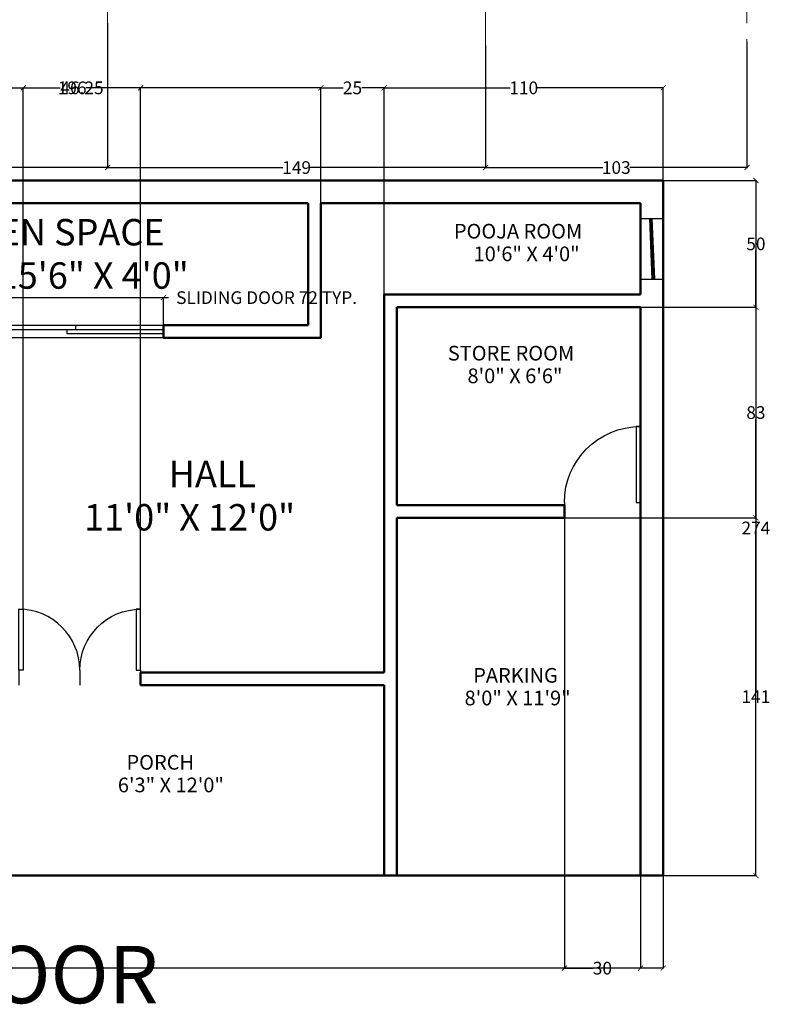
# Model space of a CAD drawing. Units: inches. Extents: x 1455 to 5994, y -182 to 2370.
# Tile 2 of 8: x 1887 to 2182, y 1415 to 1803. Entities that reach past the tile are written whole.
import ezdxf

# ---------------------------------------------------------------- set-up
doc = ezdxf.new("R2010")
doc.units = ezdxf.units.IN
doc.header["$MEASUREMENT"] = 0
doc.linetypes.add('CENTER', pattern=[50.8, 31.75, -6.35, 6.35, -6.35])
for name, color, linetype, lineweight in [('A-ANNO-DIMS', 2, 'Continuous', 18), ('A-ANNO-TEXT', 7, 'Continuous', 25), ('A-AREA-IDEN', 7, 'Continuous', 18), ('A-DOOR', 5, 'Continuous', 25), ('A-GLAZ', 4, 'Continuous', 25), ('A-GRID', 8, 'CENTER', 18), ('A-WALL', 7, 'Continuous', 50)]:
    doc.layers.add(name, color=color, linetype=linetype, lineweight=lineweight)
doc.styles.get("Standard").update_dxf_attribs({"font": 'arial.ttf'})
doc.dimstyles.get("Standard").update_dxf_attribs({"dimtxt": 5, "dimasz": 2, "dimexe": 0.18, "dimexo": 0.0625, "dimgap": 0.09, "dimtad": 0, "dimtih": 1, "dimtoh": 1, "dimdec": 1, "dimzin": 0, "dimdsep": 46, "dimlunit": 3, "dimtxsty": 'Standard', "dimblk": 'ARCHTICK', "dimcen": 0.09, "dimadec": 0, "dimazin": 0, "dimtfac": 1, "dimtdec": 1, "dimtofl": 0, "dimtmove": 0, "dimatfit": 3, "dimfxl": 1, "dimtolj": 1, "dimtzin": 0, "dimarcsym": 0})

# ---------------------------------------------------------------- blocks, each defined once
blk = doc.blocks.new('*U5')
for p, q in [((0, 0), (0, -6)), ((30, 0), (30, -6))]:
    blk.add_line(p, q)
blk.add_lwpolyline([(0, 0), (0, 30), (1.75, 30), (1.75, 0)], close=True)
blk.add_arc((0, 0), 30, 0, 90)
blk = doc.blocks.new('*U3')
for p, q in [((0, 0), (0, -6)), ((24, 0), (24, -6))]:
    blk.add_line(p, q)
blk.add_lwpolyline([(0, 0), (0, 24), (1.75, 24), (1.75, 0)], close=True)
blk.add_arc((0, 0), 24, 0, 90)
blk = doc.blocks.new('DOOR-SLIDING')
for p, q in [((37.51, 2.96), (37.51, 4.69)), ((0, 2.96), (37.51, 2.96)), ((34.07, 1.25), (34.07, 2.97)), ((72, 1.25), (34.07, 1.25)), ((37.51, 2.96), (72, 2.96))]:
    blk.add_line(p, q)
blk.add_lwpolyline([(0, 4.69), (72, 4.69), (72, -0.31), (0, -0.31)], close=True)
blk = doc.blocks.new('WIN-600')
for p, q in [((0, 0), (0, 24)), ((0.5, 0), (0.5, 24)), ((1, 0), (1, 24))]:
    blk.add_line(p, q)
blk = doc.blocks.new('_ArchTick')
at = {"color": 0, "linetype": 'ByBlock', "const_width": 0.15}
blk.add_lwpolyline([(-0.5, -0.5), (0.5, 0.5)], dxfattribs=at)
blk = doc.blocks.new('*D29')
at = {"layer": 'A-ANNO-DIMS', "color": 0, "lineweight": -2, "transparency": 16777216}
for p, q in [((1871.31, 1682.75), (1871.31, 1693.67)), ((1871.31, 1693.49), (1943.31, 1693.49)), ((1943.31, 1682.75), (1943.31, 1693.67)), ((1943.31, 1693.49), (1945.31, 1693.49))]:
    blk.add_line(p, q, dxfattribs=at)
at = {"layer": 'Defpoints', "color": 0, "lineweight": 25, "transparency": 16777216}
for p in [(1943.31, 1693.49), (1871.31, 1682.69), (1943.31, 1682.69)]:
    blk.add_point(p, dxfattribs=at)
at = {"layer": 'A-ANNO-DIMS', "color": 0, "lineweight": -2, "transparency": 16777216, "xscale": 2, "yscale": 2, "zscale": 2, "rotation": 180}
blk.add_blockref('_ArchTick', (1871.31, 1693.49), dxfattribs=at)
at = {"layer": 'A-ANNO-DIMS', "color": 0, "lineweight": -2, "transparency": 16777216, "xscale": 2, "yscale": 2, "zscale": 2}
blk.add_blockref('_ArchTick', (1943.31, 1693.49), dxfattribs=at)
at = {"layer": 'A-ANNO-DIMS', "color": 0, "transparency": 16777216, "insert": (1983.95, 1693.49), "char_height": 5, "attachment_point": 5}
blk.add_mtext('\\A1;SLIDING DOOR 72 TYP.', dxfattribs=at)
blk = doc.blocks.new('*D36')
at = {"layer": 'A-ANNO-DIMS', "color": 0, "lineweight": -2, "transparency": 16777216}
for p, q in [((1722.29, 1802.99), (1722.29, 1744.59)), ((1921.29, 1801.67), (1921.29, 1744.59)), ((1722.29, 1744.77), (1816.41, 1744.77)), ((1921.29, 1744.77), (1827.18, 1744.77))]:
    blk.add_line(p, q, dxfattribs=at)
at = {"layer": 'Defpoints', "color": 0, "lineweight": 25, "transparency": 16777216}
for p in [(1722.29, 1803.05), (1921.29, 1801.73), (1921.29, 1744.77)]:
    blk.add_point(p, dxfattribs=at)
at = {"layer": 'A-ANNO-DIMS', "color": 0, "lineweight": -2, "transparency": 16777216, "xscale": 2, "yscale": 2, "zscale": 2, "rotation": 180}
blk.add_blockref('_ArchTick', (1722.29, 1744.77), dxfattribs=at)
at = {"layer": 'A-ANNO-DIMS', "color": 0, "lineweight": -2, "transparency": 16777216, "xscale": 2, "yscale": 2, "zscale": 2}
blk.add_blockref('_ArchTick', (1921.29, 1744.77), dxfattribs=at)
at = {"layer": 'A-ANNO-DIMS', "color": 0, "transparency": 16777216, "insert": (1821.79, 1744.77), "char_height": 5, "attachment_point": 5}
blk.add_mtext('\\A1;199', dxfattribs=at)
blk = doc.blocks.new('*D37')
at = {"layer": 'A-ANNO-DIMS', "color": 0, "lineweight": -2, "transparency": 16777216}
for p, q in [((1921.29, 1801.67), (1921.29, 1744.59)), ((2070.29, 1792.96), (2070.29, 1744.59)), ((1921.29, 1744.77), (1990.41, 1744.77)), ((2070.29, 1744.77), (2001.18, 1744.77))]:
    blk.add_line(p, q, dxfattribs=at)
at = {"layer": 'Defpoints', "color": 0, "lineweight": 25, "transparency": 16777216}
for p in [(1921.29, 1801.73), (2070.29, 1793.02), (2070.29, 1744.77)]:
    blk.add_point(p, dxfattribs=at)
at = {"layer": 'A-ANNO-DIMS', "color": 0, "lineweight": -2, "transparency": 16777216, "xscale": 2, "yscale": 2, "zscale": 2, "rotation": 180}
blk.add_blockref('_ArchTick', (1921.29, 1744.77), dxfattribs=at)
at = {"layer": 'A-ANNO-DIMS', "color": 0, "lineweight": -2, "transparency": 16777216, "xscale": 2, "yscale": 2, "zscale": 2}
blk.add_blockref('_ArchTick', (2070.29, 1744.77), dxfattribs=at)
at = {"layer": 'A-ANNO-DIMS', "color": 0, "transparency": 16777216, "insert": (1995.79, 1744.77), "char_height": 5, "attachment_point": 5}
blk.add_mtext('\\A1;149', dxfattribs=at)
blk = doc.blocks.new('*D38')
at = {"layer": 'A-ANNO-DIMS', "color": 0, "lineweight": -2, "transparency": 16777216}
for p, q in [((2173.29, 1794.34), (2173.29, 1744.59)), ((2070.29, 1792.96), (2070.29, 1744.59)), ((2070.29, 1744.77), (2116.42, 1744.77)), ((2173.29, 1744.77), (2127.17, 1744.77))]:
    blk.add_line(p, q, dxfattribs=at)
at = {"layer": 'Defpoints', "color": 0, "lineweight": 25, "transparency": 16777216}
for p in [(2173.29, 1794.4), (2070.29, 1793.02), (2173.29, 1744.77)]:
    blk.add_point(p, dxfattribs=at)
at = {"layer": 'A-ANNO-DIMS', "color": 0, "lineweight": -2, "transparency": 16777216, "xscale": 2, "yscale": 2, "zscale": 2, "rotation": 180}
blk.add_blockref('_ArchTick', (2070.29, 1744.77), dxfattribs=at)
at = {"layer": 'A-ANNO-DIMS', "color": 0, "lineweight": -2, "transparency": 16777216, "xscale": 2, "yscale": 2, "zscale": 2}
blk.add_blockref('_ArchTick', (2173.29, 1744.77), dxfattribs=at)
at = {"layer": 'A-ANNO-DIMS', "color": 0, "transparency": 16777216, "insert": (2121.79, 1744.77), "char_height": 5, "attachment_point": 5}
blk.add_mtext('\\A1;103', dxfattribs=at)
blk = doc.blocks.new('*D43')
at = {"layer": 'A-ANNO-DIMS', "color": 0, "lineweight": -2, "transparency": 16777216}
for p, q in [((1551.31, 1465.62), (1551.31, 1429.01)), ((2140.31, 1465.62), (2140.31, 1429.01)), ((1551.31, 1429.19), (1840.19, 1429.19)), ((2140.31, 1429.19), (1851.43, 1429.19))]:
    blk.add_line(p, q, dxfattribs=at)
at = {"layer": 'Defpoints', "color": 0, "lineweight": 25, "transparency": 16777216}
for p in [(1551.31, 1465.69), (2140.31, 1465.69), (2140.31, 1429.19)]:
    blk.add_point(p, dxfattribs=at)
at = {"layer": 'A-ANNO-DIMS', "color": 0, "lineweight": -2, "transparency": 16777216, "xscale": 2, "yscale": 2, "zscale": 2, "rotation": 180}
blk.add_blockref('_ArchTick', (1551.31, 1429.19), dxfattribs=at)
at = {"layer": 'A-ANNO-DIMS', "color": 0, "lineweight": -2, "transparency": 16777216, "xscale": 2, "yscale": 2, "zscale": 2}
blk.add_blockref('_ArchTick', (2140.31, 1429.19), dxfattribs=at)
at = {"layer": 'A-ANNO-DIMS', "color": 0, "transparency": 16777216, "insert": (1845.81, 1429.19), "char_height": 5, "attachment_point": 5}
blk.add_mtext('\\A1;589', dxfattribs=at)
blk = doc.blocks.new('*D44')
at = {"layer": 'A-ANNO-DIMS', "color": 0, "lineweight": -2, "transparency": 16777216}
for p, q in [((2140.37, 1739.69), (2176.99, 1739.69)), ((2176.81, 1739.69), (2176.81, 1605.29)), ((2176.81, 1465.69), (2176.81, 1600.09)), ((2140.37, 1465.69), (2176.99, 1465.69))]:
    blk.add_line(p, q, dxfattribs=at)
at = {"layer": 'Defpoints', "color": 0, "lineweight": 25, "transparency": 16777216}
for p in [(2140.31, 1739.69), (2176.81, 1739.69), (2140.31, 1465.69)]:
    blk.add_point(p, dxfattribs=at)
at = {"layer": 'A-ANNO-DIMS', "color": 0, "lineweight": -2, "transparency": 16777216, "xscale": 2, "yscale": 2, "zscale": 2}
for p, rotation in [((2176.81, 1739.69), 90), ((2176.81, 1465.69), 270)]:
    blk.add_blockref('_ArchTick', p, dxfattribs=dict(at, rotation=rotation))
at = {"layer": 'A-ANNO-DIMS', "color": 0, "transparency": 16777216, "insert": (2176.81, 1602.69), "char_height": 5, "attachment_point": 5}
blk.add_mtext('\\A1;274', dxfattribs=at)
blk = doc.blocks.new('*D50')
at = {"layer": 'A-ANNO-DIMS', "color": 0, "lineweight": -2, "transparency": 16777216}
for p, q in [((1809.31, 1730.75), (1809.31, 1776.37)), ((1809.31, 1776.19), (1901.94, 1776.19)), ((2005.31, 1776.19), (1912.69, 1776.19)), ((2005.31, 1730.75), (2005.31, 1776.37))]:
    blk.add_line(p, q, dxfattribs=at)
at = {"layer": 'Defpoints', "color": 0, "lineweight": 25, "transparency": 16777216}
for p in [(2005.31, 1776.19), (1809.31, 1730.69), (2005.31, 1730.69)]:
    blk.add_point(p, dxfattribs=at)
at = {"layer": 'A-ANNO-DIMS', "color": 0, "lineweight": -2, "transparency": 16777216, "xscale": 2, "yscale": 2, "zscale": 2, "rotation": 180}
blk.add_blockref('_ArchTick', (1809.31, 1776.19), dxfattribs=at)
at = {"layer": 'A-ANNO-DIMS', "color": 0, "lineweight": -2, "transparency": 16777216, "xscale": 2, "yscale": 2, "zscale": 2}
blk.add_blockref('_ArchTick', (2005.31, 1776.19), dxfattribs=at)
at = {"layer": 'A-ANNO-DIMS', "color": 0, "transparency": 16777216, "insert": (1907.31, 1776.19), "char_height": 5, "attachment_point": 5}
blk.add_mtext('\\A1;196', dxfattribs=at)
blk = doc.blocks.new('*D51')
at = {"layer": 'A-ANNO-DIMS', "color": 0, "lineweight": -2, "transparency": 16777216}
for p, q in [((2005.31, 1730.75), (2005.31, 1776.37)), ((2005.31, 1776.19), (2014.08, 1776.19)), ((2030.31, 1776.19), (2021.54, 1776.19)), ((2030.31, 1694.75), (2030.31, 1776.37))]:
    blk.add_line(p, q, dxfattribs=at)
at = {"layer": 'Defpoints', "color": 0, "lineweight": 25, "transparency": 16777216}
for p in [(2030.31, 1776.19), (2005.31, 1730.69), (2030.31, 1694.69)]:
    blk.add_point(p, dxfattribs=at)
at = {"layer": 'A-ANNO-DIMS', "color": 0, "lineweight": -2, "transparency": 16777216, "xscale": 2, "yscale": 2, "zscale": 2, "rotation": 180}
blk.add_blockref('_ArchTick', (2005.31, 1776.19), dxfattribs=at)
at = {"layer": 'A-ANNO-DIMS', "color": 0, "lineweight": -2, "transparency": 16777216, "xscale": 2, "yscale": 2, "zscale": 2}
blk.add_blockref('_ArchTick', (2030.31, 1776.19), dxfattribs=at)
at = {"layer": 'A-ANNO-DIMS', "color": 0, "transparency": 16777216, "insert": (2017.81, 1776.19), "char_height": 5, "attachment_point": 5}
blk.add_mtext('\\A1;25', dxfattribs=at)
blk = doc.blocks.new('*D52')
at = {"layer": 'A-ANNO-DIMS', "color": 0, "lineweight": -2, "transparency": 16777216}
for p, q in [((2030.31, 1694.75), (2030.31, 1776.37)), ((2030.31, 1776.19), (2079.94, 1776.19)), ((2140.31, 1776.19), (2090.68, 1776.19)), ((2140.31, 1739.75), (2140.31, 1776.37))]:
    blk.add_line(p, q, dxfattribs=at)
at = {"layer": 'Defpoints', "color": 0, "lineweight": 25, "transparency": 16777216}
for p in [(2140.31, 1776.19), (2140.31, 1739.69), (2030.31, 1694.69)]:
    blk.add_point(p, dxfattribs=at)
at = {"layer": 'A-ANNO-DIMS', "color": 0, "lineweight": -2, "transparency": 16777216, "xscale": 2, "yscale": 2, "zscale": 2, "rotation": 180}
blk.add_blockref('_ArchTick', (2030.31, 1776.19), dxfattribs=at)
at = {"layer": 'A-ANNO-DIMS', "color": 0, "lineweight": -2, "transparency": 16777216, "xscale": 2, "yscale": 2, "zscale": 2}
blk.add_blockref('_ArchTick', (2140.31, 1776.19), dxfattribs=at)
at = {"layer": 'A-ANNO-DIMS', "color": 0, "transparency": 16777216, "insert": (2085.31, 1776.19), "char_height": 5, "attachment_point": 5}
blk.add_mtext('\\A1;110', dxfattribs=at)
blk = doc.blocks.new('*D53')
at = {"layer": 'A-ANNO-DIMS', "color": 0, "lineweight": -2, "transparency": 16777216}
for p, q in [((1560.25, 1570.69), (1514.63, 1570.69)), ((1514.81, 1570.69), (1514.81, 1520.83)), ((1514.81, 1465.69), (1514.81, 1515.54)), ((2140.25, 1465.69), (1514.63, 1465.69))]:
    blk.add_line(p, q, dxfattribs=at)
at = {"layer": 'Defpoints', "color": 0, "lineweight": 25, "transparency": 16777216}
for p in [(1514.81, 1570.69), (1560.31, 1570.69), (2140.31, 1465.69)]:
    blk.add_point(p, dxfattribs=at)
at = {"layer": 'A-ANNO-DIMS', "color": 0, "lineweight": -2, "transparency": 16777216, "xscale": 2, "yscale": 2, "zscale": 2}
for p, rotation in [((1514.81, 1570.69), 90), ((1514.81, 1465.69), 270)]:
    blk.add_blockref('_ArchTick', p, dxfattribs=dict(at, rotation=rotation))
at = {"layer": 'A-ANNO-DIMS', "color": 0, "transparency": 16777216, "insert": (1514.81, 1518.19), "char_height": 5, "attachment_point": 5}
blk.add_mtext('\\A1;105', dxfattribs=at)
blk = doc.blocks.new('*D57')
at = {"layer": 'A-ANNO-DIMS', "color": 0, "lineweight": -2, "transparency": 16777216}
for p, q in [((2035.37, 1606.69), (2176.99, 1606.69)), ((2176.81, 1606.69), (2176.81, 1538.79)), ((2176.81, 1465.69), (2176.81, 1533.59)), ((2140.37, 1465.69), (2176.99, 1465.69))]:
    blk.add_line(p, q, dxfattribs=at)
at = {"layer": 'Defpoints', "color": 0, "lineweight": 25, "transparency": 16777216}
for p in [(2035.31, 1606.69), (2176.81, 1606.69), (2140.31, 1465.69)]:
    blk.add_point(p, dxfattribs=at)
at = {"layer": 'A-ANNO-DIMS', "color": 0, "lineweight": -2, "transparency": 16777216, "xscale": 2, "yscale": 2, "zscale": 2}
for p, rotation in [((2176.81, 1606.69), 90), ((2176.81, 1465.69), 270)]:
    blk.add_blockref('_ArchTick', p, dxfattribs=dict(at, rotation=rotation))
at = {"layer": 'A-ANNO-DIMS', "color": 0, "transparency": 16777216, "insert": (2176.81, 1536.19), "char_height": 5, "attachment_point": 5}
blk.add_mtext('\\A1;141', dxfattribs=at)
blk = doc.blocks.new('*D58')
at = {"layer": 'A-ANNO-DIMS', "color": 0, "lineweight": -2, "transparency": 16777216}
for p, q in [((2035.37, 1689.69), (2176.99, 1689.69)), ((2176.81, 1689.69), (2176.81, 1650.83)), ((2176.81, 1606.69), (2176.81, 1645.54)), ((2035.37, 1606.69), (2176.99, 1606.69))]:
    blk.add_line(p, q, dxfattribs=at)
at = {"layer": 'Defpoints', "color": 0, "lineweight": 25, "transparency": 16777216}
for p in [(2035.31, 1689.69), (2176.81, 1689.69), (2035.31, 1606.69)]:
    blk.add_point(p, dxfattribs=at)
at = {"layer": 'A-ANNO-DIMS', "color": 0, "lineweight": -2, "transparency": 16777216, "xscale": 2, "yscale": 2, "zscale": 2}
for p, rotation in [((2176.81, 1689.69), 90), ((2176.81, 1606.69), 270)]:
    blk.add_blockref('_ArchTick', p, dxfattribs=dict(at, rotation=rotation))
at = {"layer": 'A-ANNO-DIMS', "color": 0, "transparency": 16777216, "insert": (2176.81, 1648.19), "char_height": 5, "attachment_point": 5}
blk.add_mtext('\\A1;83', dxfattribs=at)
blk = doc.blocks.new('*D59')
at = {"layer": 'A-ANNO-DIMS', "color": 0, "lineweight": -2, "transparency": 16777216}
for p, q in [((2140.37, 1739.69), (2176.99, 1739.69)), ((2176.81, 1739.69), (2176.81, 1717.33)), ((2176.81, 1689.69), (2176.81, 1712.04)), ((2035.37, 1689.69), (2176.99, 1689.69))]:
    blk.add_line(p, q, dxfattribs=at)
at = {"layer": 'Defpoints', "color": 0, "lineweight": 25, "transparency": 16777216}
for p in [(2140.31, 1739.69), (2176.81, 1739.69), (2035.31, 1689.69)]:
    blk.add_point(p, dxfattribs=at)
at = {"layer": 'A-ANNO-DIMS', "color": 0, "lineweight": -2, "transparency": 16777216, "xscale": 2, "yscale": 2, "zscale": 2}
for p, rotation in [((2176.81, 1739.69), 90), ((2176.81, 1689.69), 270)]:
    blk.add_blockref('_ArchTick', p, dxfattribs=dict(at, rotation=rotation))
at = {"layer": 'A-ANNO-DIMS', "color": 0, "transparency": 16777216, "insert": (2176.81, 1714.69), "char_height": 5, "attachment_point": 5}
blk.add_mtext('\\A1;50', dxfattribs=at)
blk = doc.blocks.new('*D61')
at = {"layer": 'A-ANNO-DIMS', "color": 0, "lineweight": -2, "transparency": 16777216}
for p, q in [((2101.31, 1610.87), (2101.31, 1429.01)), ((2131.31, 1612.62), (2131.31, 1429.01)), ((2101.31, 1429.19), (2112.65, 1429.19)), ((2131.31, 1429.19), (2119.97, 1429.19))]:
    blk.add_line(p, q, dxfattribs=at)
at = {"layer": 'Defpoints', "color": 0, "lineweight": 25, "transparency": 16777216}
for p in [(2101.31, 1610.94), (2131.31, 1612.69), (2131.31, 1429.19)]:
    blk.add_point(p, dxfattribs=at)
at = {"layer": 'A-ANNO-DIMS', "color": 0, "lineweight": -2, "transparency": 16777216, "xscale": 2, "yscale": 2, "zscale": 2, "rotation": 180}
blk.add_blockref('_ArchTick', (2101.31, 1429.19), dxfattribs=at)
at = {"layer": 'A-ANNO-DIMS', "color": 0, "lineweight": -2, "transparency": 16777216, "xscale": 2, "yscale": 2, "zscale": 2}
blk.add_blockref('_ArchTick', (2131.31, 1429.19), dxfattribs=at)
at = {"layer": 'A-ANNO-DIMS', "color": 0, "transparency": 16777216, "insert": (2116.31, 1429.19), "char_height": 5, "attachment_point": 5}
blk.add_mtext('\\A1;30', dxfattribs=at)
blk = doc.blocks.new('*D62')
at = {"layer": 'A-ANNO-DIMS', "color": 0, "lineweight": -2, "transparency": 16777216}
for p, q in [((1888.06, 1570.75), (1888.06, 1776.37)), ((1888.06, 1776.19), (1902.54, 1776.19)), ((1934.31, 1776.19), (1919.83, 1776.19)), ((1934.31, 1570.75), (1934.31, 1776.37))]:
    blk.add_line(p, q, dxfattribs=at)
at = {"layer": 'Defpoints', "color": 0, "lineweight": 25, "transparency": 16777216}
for p in [(1934.31, 1776.19), (1888.06, 1570.69), (1934.31, 1570.69)]:
    blk.add_point(p, dxfattribs=at)
at = {"layer": 'A-ANNO-DIMS', "color": 0, "lineweight": -2, "transparency": 16777216, "xscale": 2, "yscale": 2, "zscale": 2, "rotation": 180}
blk.add_blockref('_ArchTick', (1888.06, 1776.19), dxfattribs=at)
at = {"layer": 'A-ANNO-DIMS', "color": 0, "lineweight": -2, "transparency": 16777216, "xscale": 2, "yscale": 2, "zscale": 2}
blk.add_blockref('_ArchTick', (1934.31, 1776.19), dxfattribs=at)
at = {"layer": 'A-ANNO-DIMS', "color": 0, "transparency": 16777216, "insert": (1911.19, 1776.19), "char_height": 5, "attachment_point": 5}
blk.add_mtext('\\A1;46.25', dxfattribs=at)

msp = doc.modelspace()

# ---------------------------------------------------------------- linework, layer by layer
at = {"layer": 'A-GLAZ'}
msp.add_lwpolyline([(2131.3115, 1700.6861), (2131.3115, 1724.6861), (2140.3115, 1724.6861), (2140.3115, 1700.6861)], close=True, dxfattribs=at)
at = {"layer": 'A-GRID'}
for p, q in [((1921.2942, 2290.6569), (1921.2942, 1801.7341)), ((2070.2942, 1793.0189), (2070.2942, 2290.6569)), ((2173.2942, 2290.6569), (2173.2942, 1794.3991))]:
    msp.add_line(p, q, dxfattribs=at)
at = {"layer": 'A-WALL'}
for p, q in [((1551.3115, 1739.6861), (2140.3115, 1739.6861)), ((2140.3115, 1739.6861), (2140.3115, 1465.6861)), ((1814.3115, 1730.6861), (2000.3115, 1730.6861)), ((2000.3115, 1730.6861), (2000.3115, 1682.6861)), ((2005.3115, 1730.6861), (2030.3115, 1730.6861)), ((2005.3115, 1730.6861), (2005.3115, 1694.6861)), ((2030.3115, 1730.6861), (2131.3115, 1730.6861)), ((2131.3115, 1730.6861), (2131.3115, 1694.6861)), ((2005.3115, 1694.6861), (2005.3115, 1677.6861)), ((2030.3115, 1694.6861), (2131.3115, 1694.6861)), ((2030.3115, 1694.6861), (2030.3115, 1545.6861)), ((2035.3115, 1689.6861), (2131.3115, 1689.6861)), ((2035.3115, 1689.6861), (2035.3115, 1611.6861)), ((2131.3115, 1689.6861), (2131.3115, 1623.6861)), ((1943.3115, 1682.6861), (1943.3115, 1677.6861)), ((1943.3115, 1682.6861), (2000.3115, 1682.6861)), ((1943.3115, 1677.6861), (2005.3115, 1677.6861)), ((2131.3115, 1623.6861), (2131.3115, 1611.6861)), ((2035.3115, 1611.6861), (2101.3115, 1611.6861)), ((2101.3115, 1611.6861), (2101.3115, 1606.6861)), ((2131.3115, 1611.6861), (2131.3115, 1606.6861)), ((2035.3115, 1606.6861), (2101.3115, 1606.6861)), ((2035.3115, 1606.6861), (2035.3115, 1465.6861)), ((2131.3115, 1606.6861), (2131.3115, 1465.6861)), ((1934.3115, 1545.6861), (2030.3115, 1545.6861)), ((1934.3115, 1545.6861), (1934.3115, 1540.6861)), ((1934.3115, 1540.6861), (2030.3115, 1540.6861)), ((2030.3115, 1540.6861), (2030.3115, 1465.6861)), ((1551.3115, 1465.6861), (2035.3115, 1465.6861)), ((2035.3115, 1465.6861), (2140.3115, 1465.6861))]:
    msp.add_line(p, q, dxfattribs=at)

# ---------------------------------------------------------------- block references
at = {"layer": 'A-DOOR'}
for name, p in [('DOOR-SLIDING', (1871.312, 1678)), ('*U3', (1886.3115, 1546.6861))]:
    msp.add_blockref(name, p, dxfattribs=at)
at = {"layer": 'A-DOOR', "xscale": -1}
for name, p in [('*U5', (2131.3115, 1612.6861)), ('*U3', (1934.3115, 1546.6861))]:
    msp.add_blockref(name, p, dxfattribs=at)
at = {"layer": 'A-GLAZ', "rotation": 182.3859440303887}
msp.add_blockref('WIN-600', (2135.8111, 1724.6966), dxfattribs=at)

# ---------------------------------------------------------------- texts
at = {"layer": 'A-ANNO-TEXT'}
msp.add_text('GROUND FLOOR', height=22.629125, dxfattribs=at).set_placement((1705.5777, 1415.3353))
at = {"layer": 'A-AREA-IDEN'}
for s, height, p in [('OPEN SPACE', 10.41336, (1858.8418, 1714.0701)), ('POOJA ROOM', 5.78042, (2057.7734, 1716.7903)), ('10\'6" X 4\'0"', 5.780423, (2065.5306, 1707.8615)), ('15\'6" X 4\'0"', 10.413361, (1877.9951, 1697.0023)), ('STORE ROOM', 5.78042, (2055.3858, 1668.7036)), ('8\'0" X 6\'6"', 5.780423, (2063.143, 1659.7748)), ('HALL', 10.41336, (1945.3833, 1618.7621)), ('11\'0" X 12\'0"', 10.413361, (1912.0258, 1601.6943)), ('PARKING', 5.78042, (2065.392, 1541.7139)), ('8\'0" X 11\'9"', 5.780423, (2061.9907, 1532.785)), ('PORCH', 5.78042, (1928.7294, 1507.4336)), ('6\'3" X 12\'0"', 5.780423, (1925.3281, 1498.5047))]:
    msp.add_text(s, height=height, dxfattribs=at).set_placement(p)

# ---------------------------------------------------------------- dimensions: what is measured, and where the dimension line sits
at = {"layer": 'A-ANNO-DIMS'}
for base, p1, p2, override, picture, middle in [((1921.2942, 1744.7689), (1722.2942, 1803.0507), (1921.2942, 1801.7341), {"dimdec": 0, "dimlfac": 1, "dimrnd": 0, "dimzin": 0, "dimdsep": 46, "dimlunit": 2}, '*D36', (1821.7942, 1744.7689)), ((2070.2942, 1744.7689), (1921.2942, 1801.7341), (2070.2942, 1793.0189), {"dimdec": 0, "dimlfac": 1, "dimrnd": 0, "dimzin": 0, "dimdsep": 46, "dimlunit": 2}, '*D37', (1995.7942, 1744.7689)), ((2173.2942, 1744.7689), (2070.2942, 1793.0189), (2173.2942, 1794.3991), {"dimdec": 0, "dimlfac": 1, "dimrnd": 0, "dimzin": 0, "dimdsep": 46, "dimlunit": 2}, '*D38', (2121.7942, 1744.7689)), ((2005.3115, 1776.1861), (1809.3115, 1730.6861), (2005.3115, 1730.6861), {"dimdec": 0, "dimlfac": 1, "dimrnd": 0, "dimzin": 0, "dimdsep": 46, "dimlunit": 2}, '*D50', (1907.3115, 1776.1861)), ((1934.3115, 1776.1861), (1888.0615, 1570.6861), (1934.3115, 1570.6861), {"dimdec": 2, "dimlfac": 1, "dimrnd": 0, "dimzin": 0, "dimdsep": 46, "dimlunit": 2}, '*D62', (1911.1865, 1776.1861)), ((2030.3115, 1776.1861), (2005.3115, 1730.6861), (2030.3115, 1694.6861), {"dimdec": 0, "dimlfac": 1, "dimrnd": 0, "dimzin": 0, "dimdsep": 46, "dimlunit": 2}, '*D51', (2017.8115, 1776.1861)), ((2140.3115, 1776.1861), (2030.3115, 1694.6861), (2140.3115, 1739.6861), {"dimdec": 0, "dimlfac": 1, "dimrnd": 0, "dimzin": 0, "dimdsep": 46, "dimlunit": 2}, '*D52', (2085.3115, 1776.1861)), ((2131.3115, 1429.1861), (2101.3115, 1610.9361), (2131.3115, 1612.6861), {"dimdec": 0, "dimlfac": 1, "dimrnd": 0, "dimzin": 0, "dimdsep": 46, "dimlunit": 2}, '*D61', (2116.3115, 1429.1861)), ((2140.3115, 1429.1861), (1551.3115, 1465.6861), (2140.3115, 1465.6861), {"dimdec": 0, "dimlfac": 1, "dimrnd": 0, "dimzin": 0, "dimdsep": 46, "dimlunit": 2}, '*D43', (1845.8115, 1429.1861))]:
    dim = msp.add_linear_dim(base=base, p1=p1, p2=p2, dimstyle='Standard', override=override, dxfattribs=at)
    dim.commit()
    dim.dimension.update_dxf_attribs({"geometry": picture, "text_midpoint": middle})
for base, p1, p2, picture, middle in [((2176.8115, 1739.6861), (2035.3115, 1689.6861), (2140.3115, 1739.6861), '*D59', (2176.8115, 1714.6861)), ((2176.8115, 1739.6861), (2140.3115, 1465.6861), (2140.3115, 1739.6861), '*D44', (2176.8115, 1602.6861)), ((2176.8115, 1689.6861), (2035.3115, 1606.6861), (2035.3115, 1689.6861), '*D58', (2176.8115, 1648.1861)), ((2176.8115, 1606.6861), (2140.3115, 1465.6861), (2035.3115, 1606.6861), '*D57', (2176.8115, 1536.1861)), ((1514.8115, 1570.6861), (2140.3115, 1465.6861), (1560.3115, 1570.6861), '*D53', (1514.8115, 1518.1861))]:
    dim = msp.add_linear_dim(base=base, p1=p1, p2=p2, angle=90, dimstyle='Standard', override={"dimdec": 0, "dimlfac": 1, "dimrnd": 0, "dimzin": 0, "dimdsep": 46, "dimlunit": 2}, dxfattribs=at)
    dim.commit()
    dim.dimension.update_dxf_attribs({"geometry": picture, "text_midpoint": middle})
dim = msp.add_linear_dim(base=(1943.3115, 1693.4861), p1=(1871.3115, 1682.6861), p2=(1943.3115, 1682.6861), text='SLIDING DOOR <> TYP.', dimstyle='Standard', override={"dimdec": 0, "dimlfac": 1, "dimrnd": 0, "dimzin": 0, "dimdsep": 46, "dimlunit": 2}, dxfattribs=at)
dim.commit()
dim.dimension.update_dxf_attribs({"geometry": '*D29', "text_midpoint": (1983.9503, 1693.4861)})

doc.saveas('drawing.dxf')
